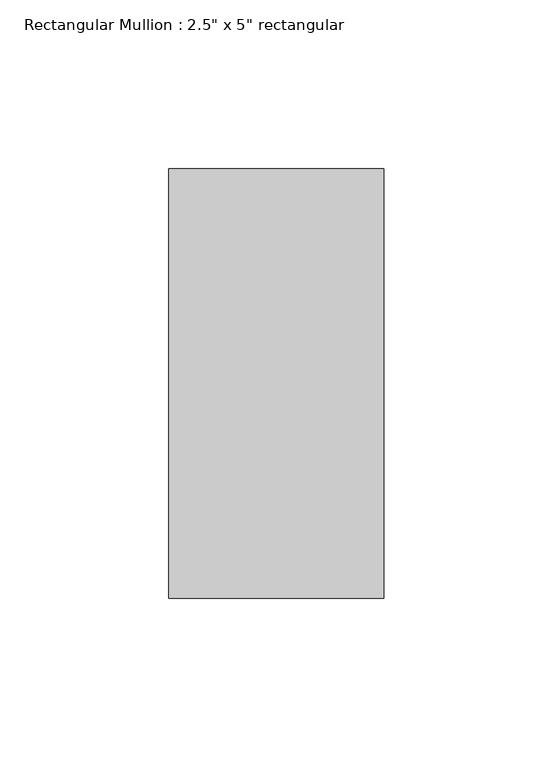
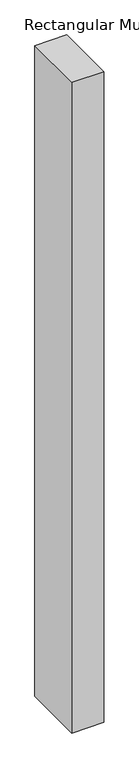
"""IFC4 building model written with IfcOpenShell, lengths in millimetres: member geometry."""

from ifc_helpers import new_model, si_unit, frame, origin, place, context, project, spatial, polyline, outline, extrude, source, transform, mapped, element, save


def member_388f8896(model_context):
    return source(origin(), model_context, "Body", "SweptSolid", [
        extrude(outline(polyline([(31.75, 63.5), (31.75, -63.5), (-31.75, -63.5), (-31.75, 63.5), (31.75, 63.5)])), frame((0.0, 0.0, -1366.313455), z_axis=(0.0, 0.0, 1.0), x_axis=(1.0, 0.0, 0.0)), (0.0, 0.0, 1.0), 1366.313455),
    ])


if __name__ == "__main__":
    model = new_model("IFC4")
    model_context = context("Model", 3, world=origin())
    ifc_project = project(units=[si_unit("LENGTHUNIT", "METRE", prefix="MILLI")], contexts=[model_context])
    site = spatial("IfcSite", under=ifc_project)
    building = spatial("IfcBuilding", under=site)
    placement = place(None, origin())
    member_shape = member_388f8896(model_context)
    element("IfcMember", 1, ObjectType="Rectangular Mullion : 2.5\" x 5\" rectangular", at=placement, inside=building, context=model_context, shape_type="MappedRepresentation", body=[
        mapped(member_shape, transform((0.0, 0.0, 0.0), x_axis=(1.0, 0.0, 0.0), y_axis=(0.0, 1.0, 0.0), z_axis=(0.0, 0.0, 1.0))),
    ])
    save(model, "model.ifc")

# Revit data of these elements
# Type "Rectangular Mullion : 2.5\" x 5\" rectangular"
#   built-in parameter 1007304 = 0.416667 (stored number, unit not read)
#   built-in parameter 1007301 = 0.104167 (stored number, unit not read)
#   built-in parameter 1007300 = 0.104167 (stored number, unit not read)
# Element 1 (IfcMember, "Rectangular Mullion : 2.5\" x 5\" rectangular")
#   Materials on its faces: "Aluminum"
# Materials
#   "Aluminum": class "Metal", colour RGB 247 247 247, transparency 0, Description = "Aluminum 6061", Cost = 0
